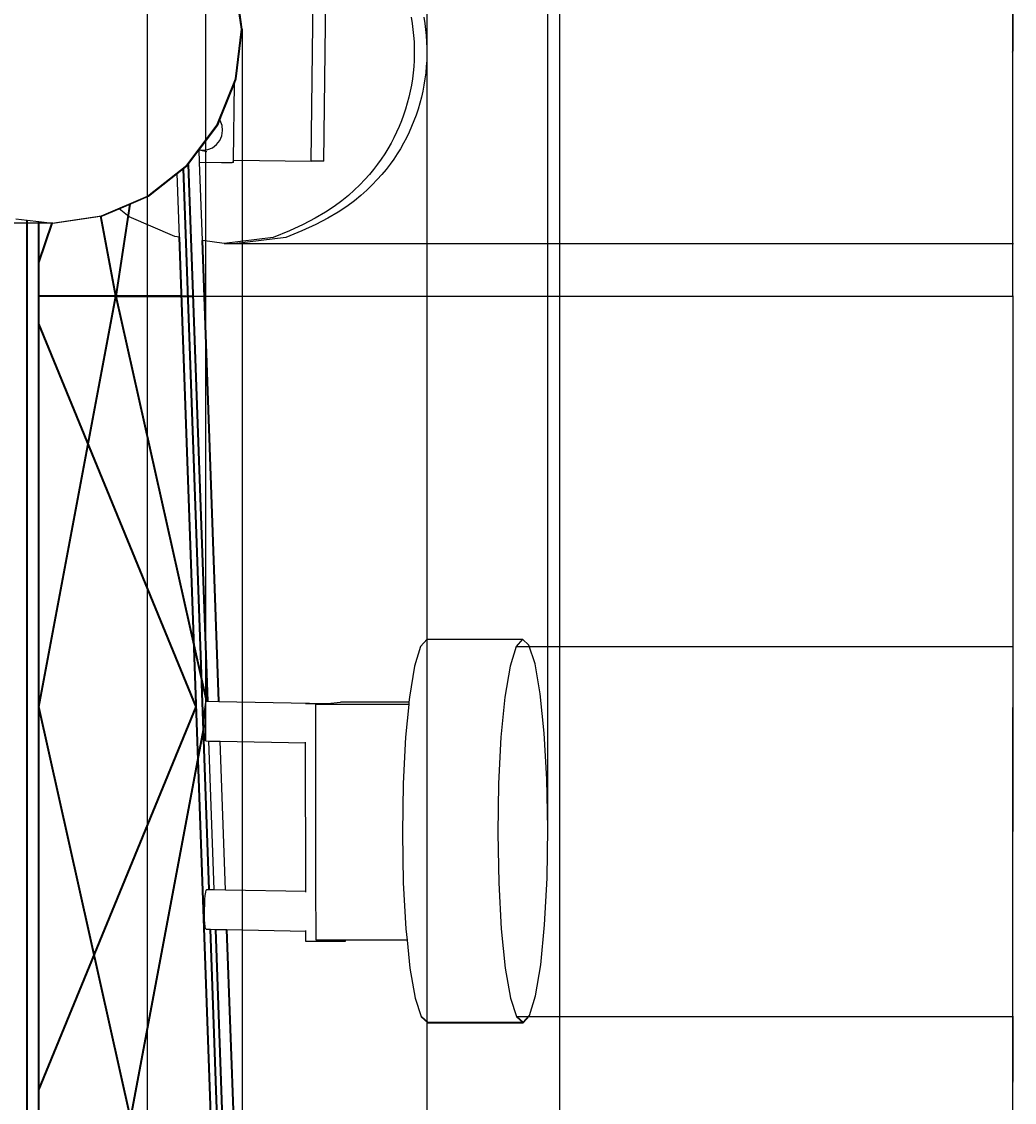
# Model space of a CAD drawing. Units: inches. Extents: x 3780 to 4301, y 1637 to 4224.
# Tile 4 of 8: x 4040 to 4301, y 3257 to 3542. Entities that reach past the tile are written whole.
import ezdxf

# ---------------------------------------------------------------- set-up
doc = ezdxf.new("R2010")
doc.units = ezdxf.units.IN
for name, color, linetype, lineweight in [('A-ANNO-DIMS', 2, 'Continuous', 18), ('E-COMM-DISH', 3, 'Continuous', 25), ('S-TOWR', 7, 'Continuous', 35)]:
    doc.layers.add(name, color=color, linetype=linetype, lineweight=lineweight)
doc.styles.get("Standard").update_dxf_attribs({"font": 'arial.ttf'})
doc.dimstyles.get("Standard").update_dxf_attribs({"dimtxt": 0.18, "dimasz": 0.18, "dimexe": 0.18, "dimexo": 0.0625, "dimgap": 0.09, "dimtad": 0, "dimtih": 1, "dimtoh": 1, "dimdec": 4, "dimzin": 0, "dimdsep": 46, "dimtxsty": 'Standard', "dimcen": 0.09, "dimadec": 0, "dimazin": 0, "dimtfac": 1, "dimtdec": 4, "dimtofl": 0, "dimtmove": 0, "dimatfit": 3, "dimfxl": 1, "dimtolj": 1, "dimtzin": 0, "dimarcsym": 0})

# ---------------------------------------------------------------- blocks, each defined once
blk = doc.blocks.new('*D20')
at = {"layer": 'A-ANNO-DIMS', "color": 0, "lineweight": -2, "transparency": 16777216}
for p, q in [((4044.72, 3469.46), (4300.89, 3469.46)), ((4300.71, 3469.28), (4300.71, 3361.65)), ((4300.71, 3253.64), (4300.71, 3361.28)), ((4044.72, 3253.46), (4300.89, 3253.46))]:
    blk.add_line(p, q, dxfattribs=at)
at = {"layer": 'A-ANNO-DIMS', "color": 0, "transparency": 16777216}
for points in [[(4300.68, 3469.28), (4300.74, 3469.28), (4300.71, 3469.46)], [(4300.68, 3253.64), (4300.74, 3253.64), (4300.71, 3253.46)]]:
    blk.add_solid(points, dxfattribs=at)
at = {"layer": 'Defpoints', "color": 0, "transparency": 16777216}
for p in [(4044.66, 3469.46), (4300.71, 3469.46), (4044.66, 3253.46)]:
    blk.add_point(p, dxfattribs=at)
at = {"layer": 'A-ANNO-DIMS', "color": 0, "transparency": 16777216, "insert": (4300.71, 3361.46), "char_height": 0.18, "attachment_point": 5}
blk.add_mtext('\\A1;216', dxfattribs=at)
blk = doc.blocks.new('*D21')
at = {"layer": 'A-ANNO-DIMS', "color": 0, "lineweight": -2, "transparency": 16777216}
for p, q in [((4010.55, 3901.46), (4300.89, 3901.46)), ((4300.71, 3901.28), (4300.71, 3685.65)), ((4300.71, 3469.64), (4300.71, 3685.28)), ((4044.72, 3469.46), (4300.89, 3469.46))]:
    blk.add_line(p, q, dxfattribs=at)
at = {"layer": 'A-ANNO-DIMS', "color": 0, "transparency": 16777216}
for points in [[(4300.68, 3901.28), (4300.74, 3901.28), (4300.71, 3901.46)], [(4300.68, 3469.64), (4300.74, 3469.64), (4300.71, 3469.46)]]:
    blk.add_solid(points, dxfattribs=at)
at = {"layer": 'Defpoints', "color": 0, "transparency": 16777216}
for p in [(4010.49, 3901.46), (4300.71, 3901.46), (4044.66, 3469.46)]:
    blk.add_point(p, dxfattribs=at)
at = {"layer": 'A-ANNO-DIMS', "color": 0, "transparency": 16777216, "insert": (4300.71, 3685.46), "char_height": 0.18, "attachment_point": 5}
blk.add_mtext('\\A1;432', dxfattribs=at)
blk = doc.blocks.new('*D22')
at = {"layer": 'A-ANNO-DIMS', "color": 0, "lineweight": -2, "transparency": 16777216}
for p, q in [((3900.05, 3694.01), (3900.05, 1636.57)), ((4181.5, 3694.01), (4181.5, 1636.57)), ((3900.23, 1636.75), (4040.31, 1636.75)), ((4181.32, 1636.75), (4041.24, 1636.75))]:
    blk.add_line(p, q, dxfattribs=at)
at = {"layer": 'A-ANNO-DIMS', "color": 0, "transparency": 16777216}
for points in [[(3900.23, 1636.78), (3900.23, 1636.72), (3900.05, 1636.75)], [(4181.32, 1636.78), (4181.32, 1636.72), (4181.5, 1636.75)]]:
    blk.add_solid(points, dxfattribs=at)
at = {"layer": 'Defpoints', "color": 0, "transparency": 16777216}
for p in [(3900.05, 3694.07), (4181.5, 3694.07), (4181.5, 1636.75)]:
    blk.add_point(p, dxfattribs=at)
at = {"layer": 'A-ANNO-DIMS', "color": 0, "transparency": 16777216, "insert": (4040.77, 1636.75), "char_height": 0.18, "attachment_point": 5}
blk.add_mtext('\\A1;281.45', dxfattribs=at)
blk = doc.blocks.new('*D27')
at = {"layer": 'A-ANNO-DIMS', "color": 0, "lineweight": -2, "transparency": 16777216}
for p, q in [((4048.31, 3488.69), (3780.66, 3488.69)), ((3780.84, 3488.51), (3780.84, 3295.31)), ((3780.84, 3101.74), (3780.84, 3294.94)), ((3926.17, 3101.56), (3780.66, 3101.56))]:
    blk.add_line(p, q, dxfattribs=at)
at = {"layer": 'A-ANNO-DIMS', "color": 0, "transparency": 16777216}
for points in [[(3780.81, 3488.51), (3780.87, 3488.51), (3780.84, 3488.69)], [(3780.81, 3101.74), (3780.87, 3101.74), (3780.84, 3101.56)]]:
    blk.add_solid(points, dxfattribs=at)
at = {"layer": 'Defpoints', "color": 0, "transparency": 16777216}
for p in [(3780.84, 3488.69), (4048.37, 3488.69), (3926.23, 3101.56)]:
    blk.add_point(p, dxfattribs=at)
at = {"layer": 'A-ANNO-DIMS', "color": 0, "transparency": 16777216, "insert": (3780.84, 3295.13), "char_height": 0.18, "attachment_point": 5}
blk.add_mtext('\\A1;387.1', dxfattribs=at)
blk = doc.blocks.new('*D28')
at = {"layer": 'A-ANNO-DIMS', "color": 0, "lineweight": -2, "transparency": 16777216}
for p, q in [((3926.17, 3691.91), (3780.66, 3691.91)), ((3780.84, 3691.73), (3780.84, 3590.48)), ((3780.84, 3488.87), (3780.84, 3590.12)), ((4048.31, 3488.69), (3780.66, 3488.69))]:
    blk.add_line(p, q, dxfattribs=at)
at = {"layer": 'A-ANNO-DIMS', "color": 0, "transparency": 16777216}
for points in [[(3780.81, 3691.73), (3780.87, 3691.73), (3780.84, 3691.91)], [(3780.81, 3488.87), (3780.87, 3488.87), (3780.84, 3488.69)]]:
    blk.add_solid(points, dxfattribs=at)
at = {"layer": 'Defpoints', "color": 0, "transparency": 16777216}
for p in [(3780.84, 3691.91), (3926.23, 3691.91), (4048.37, 3488.69)]:
    blk.add_point(p, dxfattribs=at)
at = {"layer": 'A-ANNO-DIMS', "color": 0, "transparency": 16777216, "insert": (3780.84, 3590.3), "char_height": 0.18, "attachment_point": 5}
blk.add_mtext('\\A1;203.2', dxfattribs=at)
blk = doc.blocks.new('*D42')
at = {"layer": 'A-ANNO-DIMS', "color": 0, "lineweight": -2, "transparency": 16777216}
for p, q in [((3997.15, 3538.4), (3997.15, 1636.57)), ((4098.15, 3539.64), (4098.15, 1636.57)), ((3997.33, 1636.75), (4047.38, 1636.75)), ((4097.97, 1636.75), (4047.91, 1636.75))]:
    blk.add_line(p, q, dxfattribs=at)
at = {"layer": 'A-ANNO-DIMS', "color": 0, "transparency": 16777216}
for points in [[(3997.33, 1636.78), (3997.33, 1636.72), (3997.15, 1636.75)], [(4097.97, 1636.78), (4097.97, 1636.72), (4098.15, 1636.75)]]:
    blk.add_solid(points, dxfattribs=at)
at = {"layer": 'Defpoints', "color": 0, "transparency": 16777216}
for p in [(3997.15, 3538.47), (4098.15, 3539.7), (4098.15, 1636.75)]:
    blk.add_point(p, dxfattribs=at)
at = {"layer": 'A-ANNO-DIMS', "color": 0, "transparency": 16777216, "insert": (4047.65, 1636.75), "char_height": 0.18, "attachment_point": 5}
blk.add_mtext('\\A1;101', dxfattribs=at)
blk = doc.blocks.new('*D45')
at = {"layer": 'A-ANNO-DIMS', "color": 0, "lineweight": -2, "transparency": 16777216}
for p, q in [((3971.79, 3552.9), (3780.66, 3552.9)), ((3780.84, 3552.72), (3780.84, 3520.98)), ((3780.84, 3488.87), (3780.84, 3520.61)), ((4048.31, 3488.69), (3780.66, 3488.69))]:
    blk.add_line(p, q, dxfattribs=at)
at = {"layer": 'A-ANNO-DIMS', "color": 0, "transparency": 16777216}
for points in [[(3780.81, 3552.72), (3780.87, 3552.72), (3780.84, 3552.9)], [(3780.81, 3488.87), (3780.87, 3488.87), (3780.84, 3488.69)]]:
    blk.add_solid(points, dxfattribs=at)
at = {"layer": 'Defpoints', "color": 0, "transparency": 16777216}
for p in [(3780.84, 3552.9), (3971.85, 3552.9), (4048.37, 3488.69)]:
    blk.add_point(p, dxfattribs=at)
at = {"layer": 'A-ANNO-DIMS', "color": 0, "transparency": 16777216, "insert": (3780.84, 3520.8), "char_height": 0.18, "attachment_point": 5}
blk.add_mtext('\\A1;64.21', dxfattribs=at)
blk = doc.blocks.new('*D47')
at = {"layer": 'A-ANNO-DIMS', "color": 0, "lineweight": -2, "transparency": 16777216}
for p, q in [((4094.64, 3584.08), (4300.89, 3584.08)), ((4300.71, 3583.9), (4300.71, 3533.86)), ((4300.71, 3483.47), (4300.71, 3533.5)), ((4093.42, 3483.29), (4300.89, 3483.29))]:
    blk.add_line(p, q, dxfattribs=at)
at = {"layer": 'A-ANNO-DIMS', "color": 0, "transparency": 16777216}
for points in [[(4300.68, 3583.9), (4300.74, 3583.9), (4300.71, 3584.08)], [(4300.68, 3483.47), (4300.74, 3483.47), (4300.71, 3483.29)]]:
    blk.add_solid(points, dxfattribs=at)
at = {"layer": 'Defpoints', "color": 0, "transparency": 16777216}
for p in [(4094.58, 3584.08), (4093.36, 3483.29), (4300.71, 3483.29)]:
    blk.add_point(p, dxfattribs=at)
at = {"layer": 'A-ANNO-DIMS', "color": 0, "transparency": 16777216, "insert": (4300.71, 3533.68), "char_height": 0.18, "attachment_point": 5}
blk.add_mtext('\\A1;100.79', dxfattribs=at)
blk = doc.blocks.new('*D49')
at = {"layer": 'A-ANNO-DIMS', "color": 0, "lineweight": -2, "transparency": 16777216}
for p, q in [((3999.73, 3245.63), (3999.73, 4223.96)), ((3999.91, 4223.78), (4036.16, 4223.78)), ((4073.05, 4223.78), (4036.81, 4223.78)), ((4073.23, 3245.63), (4073.23, 4223.96))]:
    blk.add_line(p, q, dxfattribs=at)
at = {"layer": 'A-ANNO-DIMS', "color": 0, "transparency": 16777216}
for points in [[(3999.91, 4223.81), (3999.91, 4223.75), (3999.73, 4223.78)], [(4073.05, 4223.81), (4073.05, 4223.75), (4073.23, 4223.78)]]:
    blk.add_solid(points, dxfattribs=at)
at = {"layer": 'Defpoints', "color": 0, "transparency": 16777216}
for p in [(4073.23, 4223.78), (3999.73, 3245.56), (4073.23, 3245.56)]:
    blk.add_point(p, dxfattribs=at)
at = {"layer": 'A-ANNO-DIMS', "color": 0, "transparency": 16777216, "insert": (4036.48, 4223.78), "char_height": 0.18, "attachment_point": 5}
blk.add_mtext('\\A1;73.5', dxfattribs=at)
blk = doc.blocks.new('*D50')
at = {"layer": 'A-ANNO-DIMS', "color": 0, "lineweight": -2, "transparency": 16777216}
for p, q in [((4073.23, 3245.63), (4073.23, 4223.96)), ((4073.41, 4223.78), (4109.66, 4223.78)), ((4146.55, 4223.78), (4110.31, 4223.78)), ((4146.73, 3245.63), (4146.73, 4223.96))]:
    blk.add_line(p, q, dxfattribs=at)
at = {"layer": 'A-ANNO-DIMS', "color": 0, "transparency": 16777216}
for points in [[(4073.41, 4223.81), (4073.41, 4223.75), (4073.23, 4223.78)], [(4146.55, 4223.81), (4146.55, 4223.75), (4146.73, 4223.78)]]:
    blk.add_solid(points, dxfattribs=at)
at = {"layer": 'Defpoints', "color": 0, "transparency": 16777216}
for p in [(4146.73, 4223.78), (4073.23, 3245.56), (4146.73, 3245.56)]:
    blk.add_point(p, dxfattribs=at)
at = {"layer": 'A-ANNO-DIMS', "color": 0, "transparency": 16777216, "insert": (4109.98, 4223.78), "char_height": 0.18, "attachment_point": 5}
blk.add_mtext('\\A1;73.5', dxfattribs=at)
blk = doc.blocks.new('*D58')
at = {"layer": 'A-ANNO-DIMS', "color": 0, "lineweight": -2, "transparency": 16777216}
for p, q in [((4170.17, 3377.39), (4300.89, 3377.39)), ((4300.71, 3377.21), (4300.71, 3328.89)), ((4300.71, 3280.21), (4300.71, 3328.53)), ((4170.32, 3280.03), (4300.89, 3280.03))]:
    blk.add_line(p, q, dxfattribs=at)
at = {"layer": 'A-ANNO-DIMS', "color": 0, "transparency": 16777216}
for points in [[(4300.68, 3377.21), (4300.74, 3377.21), (4300.71, 3377.39)], [(4300.68, 3280.21), (4300.74, 3280.21), (4300.71, 3280.03)]]:
    blk.add_solid(points, dxfattribs=at)
at = {"layer": 'Defpoints', "color": 0, "transparency": 16777216}
for p in [(4170.11, 3377.39), (4170.26, 3280.03), (4300.71, 3280.03)]:
    blk.add_point(p, dxfattribs=at)
at = {"layer": 'A-ANNO-DIMS', "color": 0, "transparency": 16777216, "insert": (4300.71, 3328.71), "char_height": 0.18, "attachment_point": 5}
blk.add_mtext('\\A1;97.35', dxfattribs=at)
blk = doc.blocks.new('*D59')
at = {"layer": 'A-ANNO-DIMS', "color": 0, "lineweight": -2, "transparency": 16777216}
for p, q in [((4088.55, 3352.58), (4088.55, 4223.96)), ((4088.73, 4223.78), (4133.13, 4223.78)), ((4178.28, 4223.78), (4133.88, 4223.78)), ((4178.46, 3329.55), (4178.46, 4223.96))]:
    blk.add_line(p, q, dxfattribs=at)
at = {"layer": 'A-ANNO-DIMS', "color": 0, "transparency": 16777216}
for points in [[(4088.73, 4223.81), (4088.73, 4223.75), (4088.55, 4223.78)], [(4178.28, 4223.81), (4178.28, 4223.75), (4178.46, 4223.78)]]:
    blk.add_solid(points, dxfattribs=at)
at = {"layer": 'Defpoints', "color": 0, "transparency": 16777216}
for p in [(4178.46, 4223.78), (4088.55, 3352.51), (4178.46, 3329.49)]:
    blk.add_point(p, dxfattribs=at)
at = {"layer": 'A-ANNO-DIMS', "color": 0, "transparency": 16777216, "insert": (4133.51, 4223.78), "char_height": 0.18, "attachment_point": 5}
blk.add_mtext('\\A1;89.91', dxfattribs=at)
blk = doc.blocks.new('*D60')
at = {"layer": 'A-ANNO-DIMS', "color": 0, "lineweight": -2, "transparency": 16777216}
for p, q in [((4170.32, 3280.03), (4300.89, 3280.03)), ((4300.71, 3279.85), (4300.71, 3262.98)), ((4300.71, 3245.74), (4300.71, 3262.62)), ((4156.54, 3245.56), (4300.89, 3245.56))]:
    blk.add_line(p, q, dxfattribs=at)
at = {"layer": 'A-ANNO-DIMS', "color": 0, "transparency": 16777216}
for points in [[(4300.68, 3279.85), (4300.74, 3279.85), (4300.71, 3280.03)], [(4300.68, 3245.74), (4300.74, 3245.74), (4300.71, 3245.56)]]:
    blk.add_solid(points, dxfattribs=at)
at = {"layer": 'Defpoints', "color": 0, "transparency": 16777216}
for p in [(4170.26, 3280.03), (4300.71, 3280.03), (4156.48, 3245.56)]:
    blk.add_point(p, dxfattribs=at)
at = {"layer": 'A-ANNO-DIMS', "color": 0, "transparency": 16777216, "insert": (4300.71, 3262.8), "char_height": 0.18, "attachment_point": 5}
blk.add_mtext('\\A1;34.47', dxfattribs=at)

msp = doc.modelspace()

# ---------------------------------------------------------------- linework, layer by layer
at = {"layer": 'E-COMM-DISH'}
for p, q in [((4116.2249, 3504.9504), (4116.9751, 3566.8887)), ((4119.6319, 3504.9504), (4120.3822, 3566.8887)), ((4097.929, 3539.6986), (4096.0526, 3552.7205)), ((4098.1498, 3539.6986), (4096.4173, 3551.7214)), ((4096.3713, 3526.6347), (4097.929, 3539.6986)), ((4096.5921, 3526.6347), (4098.1498, 3539.6986)), ((4091.4856, 3514.4192), (4096.3713, 3526.6347)), ((4096.0985, 3525.4007), (4096.5921, 3526.6347)), ((4092.7821, 3517.1087), (4096.0985, 3525.4007)), ((4095.8538, 3505.2014), (4096.0985, 3525.4007)), ((4091.7064, 3514.4192), (4092.2335, 3515.7372)), ((4092.2335, 3515.7372), (4092.7821, 3517.1087)), ((4092.3246, 3515.615), (4092.2335, 3515.7372)), ((4092.828, 3514.3505), (4092.3246, 3515.615)), ((4083.6049, 3503.8844), (4091.4856, 3514.4192)), ((4087.2109, 3508.4097), (4091.7064, 3514.4192)), ((4092.794, 3511.6488), (4092.9881, 3512.9977)), ((4092.9881, 3512.9977), (4092.828, 3514.3505)), ((4091.4193, 3509.3239), (4092.2589, 3510.3957)), ((4092.2589, 3510.3957), (4092.794, 3511.6488)), ((4083.9726, 3504.0807), (4086.8364, 3507.9091)), ((4086.8364, 3507.9091), (4086.855, 3507.9339)), ((4086.9514, 3504.6745), (4086.8364, 3507.9091)), ((4086.855, 3507.9339), (4086.8728, 3507.9577)), ((4086.855, 3507.9339), (4088.818, 3507.5433)), ((4086.8728, 3507.9577), (4087.2109, 3508.4097)), ((4086.8728, 3507.9577), (4087.7245, 3507.8356)), ((4087.7245, 3507.8356), (4088.0588, 3507.876)), ((4088.0588, 3507.876), (4089.0721, 3507.9986)), ((4089.0721, 3507.9986), (4090.3323, 3508.5063)), ((4090.3323, 3508.5063), (4091.4193, 3509.3239)), ((4073.2662, 3495.7484), (4083.6049, 3503.8844)), ((4082.7117, 3503.0077), (4083.8257, 3503.8844)), ((4083.8257, 3503.8844), (4083.9726, 3504.0807)), ((4087.6827, 3484.1131), (4086.9514, 3504.6745)), ((4086.9514, 3504.6745), (4092.6684, 3504.6033)), ((4092.6684, 3504.6033), (4095.4935, 3504.5736)), ((4095.8462, 3504.5714), (4095.4935, 3504.5736)), ((4095.8462, 3504.5714), (4095.8538, 3505.2014)), ((4095.8538, 3505.2014), (4116.2249, 3504.9504)), ((4119.6319, 3504.9504), (4116.2249, 3504.9504)), ((4073.487, 3495.7484), (4081.057, 3501.7056)), ((4081.057, 3501.7056), (4082.7117, 3503.0077)), ((4081.6516, 3484.9897), (4081.057, 3501.7056)), ((4061.1741, 3490.5655), (4073.2662, 3495.7484)), ((4065.8038, 3492.4552), (4073.487, 3495.7484)), ((4061.3949, 3490.5655), (4065.8038, 3492.4552)), ((4068.4595, 3490.3474), (4065.8038, 3492.4552)), ((4038.6622, 3489.8207), (4041.6622, 3489.463)), ((4048.1527, 3488.689), (4061.1741, 3490.5655)), ((4048.3735, 3488.689), (4061.3949, 3490.5655)), ((4080.4485, 3485.1646), (4068.4595, 3490.3474)), ((4041.6622, 3489.463), (4044.6622, 3489.1052)), ((4044.6622, 3489.1052), (4048.1527, 3488.689)), ((4048.3735, 3488.689), (4048.1527, 3488.689)), ((4081.6516, 3484.9897), (4080.4485, 3485.1646)), ((4093.359, 3483.2881), (4087.6827, 3484.1131)), ((4106.3112, 3484.8459), (4093.359, 3483.2881)), ((4109.6134, 3484.8459), (4096.6613, 3483.2881)), ((4093.359, 3483.2881), (4096.6613, 3483.2881)), ((4146.7222, 3379.264), (4145.0225, 3377.3875)), ((4146.7222, 3379.264), (4171.805, 3379.264)), ((4171.805, 3379.264), (4170.1053, 3377.3875)), ((4173.5102, 3377.7062), (4171.805, 3379.264)), ((4145.0225, 3377.3875), (4143.4441, 3372.2047)), ((4170.1053, 3377.3875), (4168.5269, 3372.2047)), ((4175.1046, 3372.8204), (4173.5102, 3377.7062)), ((4143.4441, 3372.2047), (4142.0946, 3364.0686)), ((4168.5269, 3372.2047), (4167.1774, 3364.0686)), ((4176.4797, 3364.9394), (4175.1046, 3372.8204)), ((4177.5416, 3354.6003), (4176.4797, 3364.9394)), ((4088.3655, 3361.3836), (4088.4792, 3362.2249)), ((4088.4792, 3362.2249), (4088.604, 3362.7601)), ((4088.604, 3362.7601), (4088.7315, 3362.9527)), ((4088.7315, 3362.9527), (4088.9921, 3362.9479)), ((4088.9921, 3362.9479), (4091.9941, 3362.8928)), ((4091.9941, 3362.8928), (4120.5511, 3362.3687)), ((4115.1136, 3362.2634), (4114.7902, 3362.2775)), ((4115.795, 3362.2502), (4115.1136, 3362.2634)), ((4116.7587, 3362.2401), (4115.795, 3362.2502)), ((4117.9389, 3362.2337), (4116.7587, 3362.2401)), ((4117.4462, 3362.0768), (4119.1013, 3362.2318)), ((4141.9001, 3362.0768), (4117.4462, 3362.0768)), ((4117.4512, 3358.9859), (4117.4462, 3362.0768)), ((4119.1013, 3362.2318), (4117.9389, 3362.2337)), ((4119.1013, 3362.2318), (4119.7046, 3362.2882)), ((4119.7046, 3362.2882), (4120.5502, 3362.3674)), ((4120.5502, 3362.3674), (4120.5511, 3362.3687)), ((4120.5511, 3362.3687), (4123.9977, 3362.6901)), ((4120.5511, 3362.3687), (4120.552, 3362.3676)), ((4141.96, 3362.6901), (4123.9977, 3362.6901)), ((4141.9001, 3362.0768), (4141.0659, 3353.5339)), ((4141.96, 3362.6901), (4141.9001, 3362.0768)), ((4142.0946, 3364.0686), (4141.96, 3362.6901)), ((4167.1774, 3364.0686), (4166.1487, 3353.5339)), ((4088.1613, 3357.6763), (4088.2009, 3359.0291)), ((4088.2009, 3359.0291), (4088.2705, 3360.2936)), ((4088.2705, 3360.2936), (4088.3655, 3361.3836)), ((4117.457, 3355.2899), (4117.4512, 3358.9859)), ((4088.1544, 3356.3274), (4088.1613, 3357.6763)), ((4088.1808, 3355.0743), (4088.1544, 3356.3274)), ((4088.2386, 3354.0025), (4088.1808, 3355.0743)), ((4088.3238, 3353.1848), (4088.2386, 3354.0025)), ((4088.4307, 3352.6772), (4088.3238, 3353.1848)), ((4117.5301, 3309.4955), (4117.457, 3355.2899)), ((4141.0659, 3353.5339), (4140.4282, 3341.3183)), ((4166.1487, 3353.5339), (4165.511, 3341.3183)), ((4178.2181, 3342.5078), (4177.5416, 3354.6003)), ((4088.552, 3352.5141), (4088.4307, 3352.6772)), ((4088.552, 3352.5141), (4089.3637, 3352.4992)), ((4090.7534, 3313.4267), (4089.3637, 3352.4992)), ((4089.3637, 3352.4992), (4092.3657, 3352.4442)), ((4093.7554, 3313.3716), (4092.3657, 3352.4442)), ((4092.3657, 3352.4442), (4114.7772, 3352.0328)), ((4114.7772, 3352.0328), (4114.777, 3352.1801)), ((4114.8395, 3312.9846), (4114.7772, 3352.0328)), ((4178.4631, 3329.4859), (4178.2181, 3342.5078)), ((4140.4282, 3341.3183), (4140.2249, 3328.2544)), ((4165.511, 3341.3183), (4165.3076, 3328.2544)), ((4140.2249, 3328.2544), (4140.4698, 3315.2325)), ((4165.3076, 3328.2544), (4165.5526, 3315.2325)), ((4178.2597, 3316.422), (4178.4631, 3329.4859)), ((4177.622, 3304.2064), (4178.2597, 3316.422)), ((4088.683, 3313.2697), (4088.8104, 3313.4623)), ((4088.8104, 3313.4623), (4089.4535, 3313.4505)), ((4089.4535, 3313.4505), (4090.7534, 3313.4267)), ((4090.7534, 3313.4267), (4093.7554, 3313.3716)), ((4093.7554, 3313.3716), (4114.8395, 3312.9846)), ((4140.4698, 3315.2325), (4141.1463, 3303.14)), ((4165.5526, 3315.2325), (4166.2291, 3303.14)), ((4088.2798, 3309.5387), (4088.3494, 3310.8032)), ((4088.3494, 3310.8032), (4088.4444, 3311.8932)), ((4088.4444, 3311.8932), (4088.5581, 3312.7345)), ((4088.5581, 3312.7345), (4088.683, 3313.2697)), ((4114.8398, 3312.8043), (4114.8395, 3312.9846)), ((4088.2334, 3306.837), (4088.2402, 3308.1859)), ((4088.2402, 3308.1859), (4088.2798, 3309.5387)), ((4117.536, 3305.7995), (4117.5301, 3309.4955)), ((4088.2597, 3305.5839), (4088.2334, 3306.837)), ((4088.3175, 3304.5121), (4088.2597, 3305.5839)), ((4117.545, 3300.1385), (4117.536, 3305.7995)), ((4088.4027, 3303.6944), (4088.3175, 3304.5121)), ((4088.5096, 3303.1868), (4088.4027, 3303.6944)), ((4088.6309, 3303.0237), (4088.5096, 3303.1868)), ((4088.6309, 3303.0237), (4089.8251, 3303.0018)), ((4089.8251, 3303.0018), (4091.125, 3302.978)), ((4091.125, 3302.978), (4094.127, 3302.9229)), ((4094.127, 3302.9229), (4114.8562, 3302.5424)), ((4114.8562, 3302.5424), (4114.8559, 3302.6897)), ((4114.8605, 3299.8069), (4114.8562, 3302.5424)), ((4141.1463, 3303.14), (4141.4546, 3300.1385)), ((4166.2291, 3303.14), (4167.291, 3292.8009)), ((4176.5933, 3293.6717), (4177.622, 3304.2064)), ((4115.2132, 3299.7915), (4114.8605, 3299.8069)), ((4115.8947, 3299.7783), (4115.2132, 3299.7915)), ((4116.8583, 3299.7682), (4115.8947, 3299.7783)), ((4118.0386, 3299.7618), (4116.8583, 3299.7682)), ((4125.2116, 3300.1385), (4117.545, 3300.1385)), ((4119.355, 3299.7596), (4118.0386, 3299.7618)), ((4120.7178, 3299.7618), (4119.355, 3299.7596)), ((4122.0341, 3299.7682), (4120.7178, 3299.7618)), ((4123.2144, 3299.7783), (4122.0341, 3299.7682)), ((4124.178, 3299.7915), (4123.2144, 3299.7783)), ((4124.8594, 3299.8069), (4124.178, 3299.7915)), ((4125.2121, 3299.8234), (4124.8594, 3299.8069)), ((4141.4546, 3300.1385), (4125.2116, 3300.1385)), ((4125.2116, 3300.1385), (4125.2121, 3299.8234)), ((4141.4546, 3300.1385), (4142.2082, 3292.8009)), ((4175.2438, 3285.5356), (4176.5933, 3293.6717)), ((4142.2082, 3292.8009), (4143.5833, 3284.9199)), ((4167.291, 3292.8009), (4168.6661, 3284.9199)), ((4143.5833, 3284.9199), (4145.1778, 3280.034)), ((4168.6661, 3284.9199), (4170.2605, 3280.034)), ((4173.6654, 3280.3528), (4175.2438, 3285.5356))]:
    msp.add_line(p, q, dxfattribs=at)
for points in [[(4142.533, 3542.8046), (4142.8028, 3541.197), (4143.0203, 3539.5814), (4143.1855, 3537.9595), (4143.2981, 3536.333), (4143.3579, 3534.7036), (4143.3648, 3533.0732), (4143.3184, 3531.4435), (4143.2192, 3529.8161), (4143.0672, 3528.1929), (4142.8628, 3526.5755), (4142.6062, 3524.9657), (4142.2976, 3523.3653), (4141.9372, 3521.7759), (4141.5255, 3520.1992), (4141.0625, 3518.6371), (4140.5491, 3517.0911), (4139.9857, 3515.5629), (4139.3732, 3514.054), (4138.7123, 3512.566), (4138.0035, 3511.1007), (4137.2476, 3509.6595), (4136.4453, 3508.2441), (4135.5956, 3506.8547), (4134.691, 3505.4865), (4133.7224, 3504.133), (4132.6807, 3502.7879), (4131.5568, 3501.445), (4130.3414, 3500.0978), (4129.0256, 3498.7402), (4127.6001, 3497.3657), (4126.0464, 3495.9677), (4124.308, 3494.5384), (4122.3192, 3493.0695), (4120.0139, 3491.5529), (4117.3264, 3489.9805), (4114.1906, 3488.3439), (4110.5409, 3486.6351), (4106.3112, 3484.8459)], [(4145.8352, 3542.8046), (4146.105, 3541.197), (4146.3225, 3539.5814), (4146.4877, 3537.9595), (4146.6003, 3536.333), (4146.6601, 3534.7036), (4146.667, 3533.0732), (4146.6207, 3531.4435), (4146.5214, 3529.8161), (4146.3694, 3528.1929), (4146.165, 3526.5755), (4145.9084, 3524.9657), (4145.5998, 3523.3653), (4145.2394, 3521.7759), (4144.8277, 3520.1992), (4144.3647, 3518.6371), (4143.8513, 3517.0911), (4143.2879, 3515.5629), (4142.6755, 3514.054), (4142.0145, 3512.566), (4141.3057, 3511.1007), (4140.5498, 3509.6595), (4139.7475, 3508.2441), (4138.8978, 3506.8547), (4137.9932, 3505.4865), (4137.0246, 3504.133), (4135.9829, 3502.7879), (4134.859, 3501.445), (4133.6436, 3500.0978), (4132.3278, 3498.7402), (4130.9023, 3497.3657), (4129.3486, 3495.9677), (4127.6103, 3494.5384), (4125.6214, 3493.0695), (4123.3161, 3491.5529), (4120.6286, 3489.9805), (4117.4929, 3488.3439), (4113.8431, 3486.6351), (4109.6134, 3484.8459)]]:
    msp.add_lwpolyline(points, dxfattribs=at)
at = {"layer": 'S-TOWR'}
for p, q in [((4083.9726, 3504.0807), (4088.9921, 3362.9479)), ((4089.4535, 3313.4505), (4082.7117, 3503.0077)), ((4068.6137, 3493.6596), (4064.933, 3469.4644)), ((4064.933, 3469.4644), (4060.9836, 3490.5062)), ((4041.6622, 3173.2144), (4041.6622, 3489.463)), ((4044.6622, 3179.2144), (4044.6622, 3489.1052)), ((4044.6622, 3478.2927), (4048.1951, 3488.689)), ((4089.8594, 3254.2144), (4081.6516, 3484.9897)), ((4091.9941, 3362.8928), (4087.6827, 3484.1131)), ((4082.2037, 3469.4644), (4044.6622, 3469.4644)), ((4044.6622, 3361.4644), (4064.933, 3469.4644)), ((4064.933, 3469.4644), (4085.2037, 3469.4644)), ((4064.933, 3469.4644), (4088.7174, 3362.9314)), ((4086.0449, 3361.4644), (4044.6622, 3462.1643)), ((4044.6622, 3260.7646), (4086.0449, 3361.4644)), ((4068.7741, 3253.4644), (4044.6622, 3361.4644)), ((4088.1565, 3356.7311), (4068.7741, 3253.4644)), ((4094.3345, 3176.2144), (4089.8251, 3303.0018)), ((4091.125, 3302.978), (4095.6335, 3176.2144)), ((4096.167, 3245.5639), (4094.127, 3302.9229)), ((4145.1778, 3280.034), (4146.8829, 3278.4763)), ((4170.2605, 3280.034), (4171.9657, 3278.4763)), ((4171.9657, 3278.4763), (4173.6654, 3280.3528)), ((4146.8829, 3278.4763), (4171.9657, 3278.4763))]:
    msp.add_line(p, q, dxfattribs=at)

# ---------------------------------------------------------------- dimensions: what is measured, and where the dimension line sits
at = {"layer": 'A-ANNO-DIMS'}
for base, p1, p2, override, picture, middle in [((4073.2315, 4223.7769), (3999.7315, 3245.5639), (4073.2315, 3245.5639), {"dimdec": 1, "dimlfac": 1, "dimrnd": 0, "dimzin": 0, "dimdsep": 46, "dimlunit": 2}, '*D49', (4036.4815, 4223.7769)), ((4146.7315, 4223.7769), (4073.2315, 3245.5639), (4146.7315, 3245.5639), {"dimdec": 1, "dimlfac": 1, "dimrnd": 0, "dimzin": 0, "dimdsep": 46, "dimlunit": 2}, '*D50', (4109.9815, 4223.7769)), ((4178.4631, 4223.7769), (4088.552, 3352.5141), (4178.4631, 3329.4859), {"dimdec": 2, "dimlfac": 1, "dimrnd": 0, "dimzin": 0, "dimdsep": 46, "dimlunit": 2}, '*D59', (4133.5075, 4223.7769)), ((4181.498, 1636.7487), (3900.0482, 3694.0677), (4181.498, 3694.0677), {"dimdec": 2, "dimlfac": 1, "dimrnd": 0, "dimzin": 0, "dimdsep": 46, "dimlunit": 2}, '*D22', (4040.7731, 1636.7487)), ((4098.1498, 1636.7487), (3997.1451, 3538.4672), (4098.1498, 3539.6986), {"dimdec": 0, "dimlfac": 1, "dimrnd": 0, "dimzin": 0, "dimdsep": 46, "dimlunit": 2}, '*D42', (4047.6474, 1636.7487))]:
    dim = msp.add_linear_dim(base=base, p1=p1, p2=p2, dimstyle='Standard', override=override, dxfattribs=at)
    dim.commit()
    dim.dimension.update_dxf_attribs({"geometry": picture, "text_midpoint": middle})
for base, p1, p2, override, picture, middle in [((4300.7091, 3901.4644), (4044.6622, 3469.4644), (4010.4853, 3901.4644), {"dimdec": 0, "dimlfac": 1, "dimrnd": 0, "dimzin": 0, "dimdsep": 46, "dimlunit": 2}, '*D21', (4300.7091, 3685.4644)), ((3780.8371, 3691.9077), (4048.3735, 3488.689), (3926.2315, 3691.9077), {"dimdec": 1, "dimlfac": 1, "dimrnd": 0, "dimzin": 0, "dimdsep": 46, "dimlunit": 2}, '*D28', (3780.8371, 3590.2983)), ((4300.7091, 3483.2881), (4094.5799, 3584.0758), (4093.359, 3483.2881), {"dimdec": 2, "dimlfac": 1, "dimrnd": 0, "dimzin": 0, "dimdsep": 46, "dimlunit": 2}, '*D47', (4300.7091, 3533.682)), ((3780.8371, 3552.903), (4048.3735, 3488.689), (3971.8516, 3552.903), {"dimdec": 2, "dimlfac": 1, "dimrnd": 0, "dimzin": 0, "dimdsep": 46, "dimlunit": 2}, '*D45', (3780.8371, 3520.796)), ((3780.8371, 3488.689), (3926.2315, 3101.5639), (4048.3735, 3488.689), {"dimdec": 1, "dimlfac": 1, "dimrnd": 0, "dimzin": 0, "dimdsep": 46, "dimlunit": 2}, '*D27', (3780.8371, 3295.1265)), ((4300.7091, 3469.4644), (4044.6622, 3253.4644), (4044.6622, 3469.4644), {"dimdec": 0, "dimlfac": 1, "dimrnd": 0, "dimzin": 0, "dimdsep": 46, "dimlunit": 2}, '*D20', (4300.7091, 3361.4644)), ((4300.7091, 3280.034), (4170.1053, 3377.3875), (4170.2605, 3280.034), {"dimdec": 2, "dimlfac": 1, "dimrnd": 0, "dimzin": 0, "dimdsep": 46, "dimlunit": 2}, '*D58', (4300.7091, 3328.7108)), ((4300.7091, 3280.034), (4156.4815, 3245.5639), (4170.2605, 3280.034), {"dimdec": 2, "dimlfac": 1, "dimrnd": 0, "dimzin": 0, "dimdsep": 46, "dimlunit": 2}, '*D60', (4300.7091, 3262.799))]:
    dim = msp.add_linear_dim(base=base, p1=p1, p2=p2, angle=90, dimstyle='Standard', override=override, dxfattribs=at)
    dim.commit()
    dim.dimension.update_dxf_attribs({"geometry": picture, "text_midpoint": middle})

doc.saveas('drawing.dxf')
